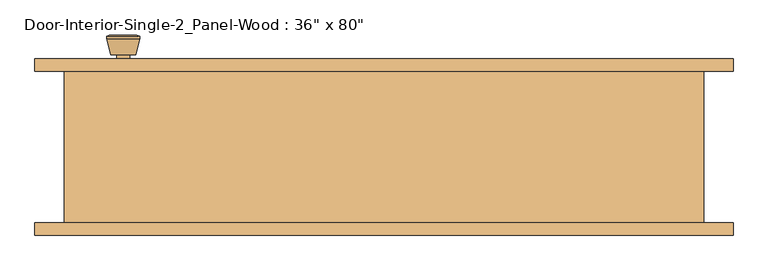
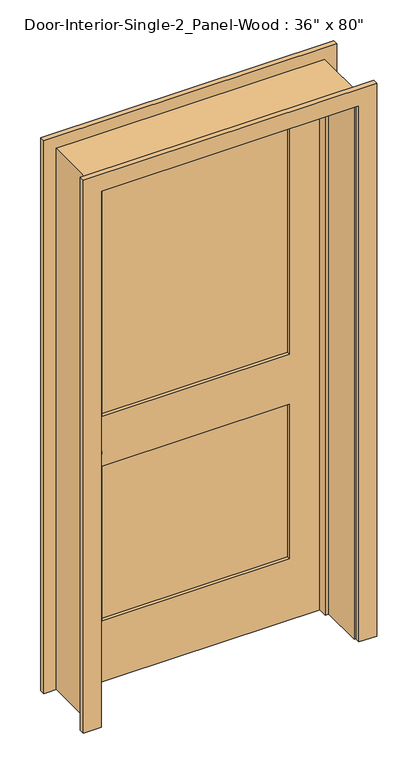
"""IFC4 building model written with IfcOpenShell, lengths in millimetres: door geometry."""

from ifc_helpers import new_model, si_unit, point, frame, frame_2d, origin, place, context, project, spatial, polyline, circle_curve, trimmed, segment, composite_curve, outline, extrude, faceted_brep, source, transform, mapped, element, save
from ifc_brep_helpers import plane_surface, cylinder_surface, revolved_surface, advanced_brep


def door_18b56f29(model_context):
    return source(origin(), model_context, "Body", "SolidModel", [
        advanced_brep(
        [(-393.7, 70.2, 914.4), (-383.7, 70.2, 914.4), (-403.7, 70.2, 914.4), (-373.2241324, 21.2, 914.4), (-393.7, 21.2, 914.4), (-414.1758676, 21.2, 914.4), (-368.7, 23.0278681, 914.4), (-418.7, 23.0278681, 914.4), (-368.7, 26.4915463, 914.4), (-418.7, 26.4915463, 914.4), (-375.063764, 51.2, 914.4), (-412.336236, 51.2, 914.4), (-383.7, 51.2, 914.4), (-403.7, 51.2, 914.4)],
        [
            (0, 1),
            (1, 2, circle_curve(frame((-393.7, 70.2, 914.4), z_axis=(0.0, 1.0, 0.0), x_axis=(-1.0, 0.0, 0.0)), 10.0)),
            (2, 0),
            (2, 1, circle_curve(frame((-393.7, 70.2, 914.4), z_axis=(0.0, 1.0, 0.0), x_axis=(-1.0, 0.0, 0.0)), 10.0)),
            (3, 4),
            (4, 5),
            (5, 3, circle_curve(frame((-393.7, 21.2, 914.4), z_axis=(0.0, -1.0, 0.0), x_axis=(-1.0, 0.0, 0.0)), 20.4758676)),
            (3, 5, circle_curve(frame((-393.7, 21.2, 914.4), z_axis=(0.0, -1.0, 0.0), x_axis=(-1.0, 0.0, 0.0)), 20.4758676)),
            (6, 3),
            (5, 7),
            (7, 6, circle_curve(frame((-393.7, 23.0278681, 914.4), z_axis=(0.0, -1.0, 0.0), x_axis=(-1.0, 0.0, 0.0)), 25.0)),
            (6, 7, circle_curve(frame((-393.7, 23.0278681, 914.4), z_axis=(0.0, -1.0, 0.0), x_axis=(-1.0, 0.0, 0.0)), 25.0)),
            (8, 6),
            (7, 9),
            (9, 8, circle_curve(frame((-393.7, 26.4915463, 914.4), z_axis=(0.0, -1.0, 0.0), x_axis=(-1.0, 0.0, 0.0)), 25.0)),
            (8, 9, circle_curve(frame((-393.7, 26.4915463, 914.4), z_axis=(0.0, -1.0, 0.0), x_axis=(-1.0, 0.0, 0.0)), 25.0)),
            (10, 8),
            (9, 11),
            (11, 10, circle_curve(frame((-393.7, 51.2, 914.4), z_axis=(0.0, -1.0, 0.0), x_axis=(-1.0, 0.0, 0.0)), 18.636236)),
            (10, 11, circle_curve(frame((-393.7, 51.2, 914.4), z_axis=(0.0, -1.0, 0.0), x_axis=(-1.0, 0.0, 0.0)), 18.636236)),
            (12, 10),
            (11, 13),
            (13, 12, circle_curve(frame((-393.7, 51.2, 914.4), z_axis=(0.0, -1.0, 0.0), x_axis=(-1.0, 0.0, 0.0)), 10.0)),
            (12, 13, circle_curve(frame((-393.7, 51.2, 914.4), z_axis=(0.0, -1.0, 0.0), x_axis=(-1.0, 0.0, 0.0)), 10.0)),
            (1, 12),
            (13, 2),
        ],
        [
            plane_surface(frame((-393.7, 70.2, 914.4), z_axis=(0.0, 1.0, 0.0), x_axis=(-1.0, 0.0, 0.0))),
            plane_surface(frame((-393.7, 21.2, 914.4), z_axis=(0.0, -1.0, 0.0), x_axis=(-1.0, 0.0, 0.0))),
            revolved_surface(polyline([(-414.1758676, 21.2, 914.4), (-418.7, 23.0278681, 914.4)]), (-393.7, 70.2, 914.4), (0.0, 1.0, 0.0)),
            cylinder_surface(frame((-393.7, 70.2, 914.4), z_axis=(0.0, 1.0, 0.0), x_axis=(-1.0, 0.0, 0.0)), 25.0),
            revolved_surface(polyline([(-418.7, 26.4915463, 914.4), (-412.336236, 51.2, 914.4)]), (-393.7, 70.2, 914.4), (0.0, 1.0, 0.0)),
            plane_surface(frame((-393.7, 51.2, 914.4), z_axis=(0.0, 1.0, 0.0), x_axis=(-1.0, 0.0, 0.0))),
            cylinder_surface(frame((-393.7, 70.2, 914.4), z_axis=(0.0, 1.0, 0.0), x_axis=(-1.0, 0.0, 0.0)), 10.0),
        ],
        [
            (0, [[1, 2, 3]]),
            (0, [[-3, 4, -1]]),
            (1, [[5, 6, 7]]),
            (1, [[-6, -5, 8]]),
            (2, [[9, -7, 10, 11]]),
            (2, [[-10, -8, -9, 12]]),
            (3, [[13, -11, 14, 15]]),
            (3, [[-14, -12, -13, 16]]),
            (4, [[17, -15, 18, 19]]),
            (4, [[-18, -16, -17, 20]]),
            (5, [[21, -19, 22, 23]]),
            (5, [[-22, -20, -21, 24]]),
            (6, [[25, -23, 26, -2]]),
            (6, [[-26, -24, -25, -4]]),
        ],
    ),
        extrude(outline(composite_curve([segment(trimmed(circle_curve(frame_2d((914.4, -393.7)), 30.0), [point((914.4, -423.7))], [point((914.4, -363.7))], False, "CARTESIAN"), True, "CONTINUOUS"), segment(trimmed(circle_curve(frame_2d((914.4, -393.7)), 30.0), [point((914.4, -363.7))], [point((914.4, -423.7))], False, "CARTESIAN"), True, "CONTINUOUS")], self_intersect=False)), frame((0.0, 70.2, 0.0), z_axis=(0.0, 1.0, 0.0), x_axis=(0.0, 0.0, 1.0)), (0.0, 0.0, 1.0), 6.0),
        advanced_brep(
        [(-393.7, 117.125, 914.4), (-403.7, 117.125, 914.4), (-383.7, 117.125, 914.4), (-373.2241324, 166.125, 914.4), (-414.1758676, 166.125, 914.4), (-393.7, 166.125, 914.4), (-368.7, 164.2971319, 914.4), (-418.7, 164.2971319, 914.4), (-368.7, 160.8334537, 914.4), (-418.7, 160.8334537, 914.4), (-375.063764, 136.125, 914.4), (-412.336236, 136.125, 914.4), (-383.7, 136.125, 914.4), (-403.7, 136.125, 914.4)],
        [
            (0, 1),
            (1, 2, circle_curve(frame((-393.7, 117.125, 914.4), z_axis=(0.0, -1.0, 0.0), x_axis=(-1.0, 0.0, 0.0)), 10.0)),
            (2, 0),
            (2, 1, circle_curve(frame((-393.7, 117.125, 914.4), z_axis=(0.0, -1.0, 0.0), x_axis=(-1.0, 0.0, 0.0)), 10.0)),
            (3, 4, circle_curve(frame((-393.7, 166.125, 914.4), z_axis=(0.0, 1.0, 0.0), x_axis=(-1.0, 0.0, 0.0)), 20.4758676)),
            (4, 5),
            (5, 3),
            (4, 3, circle_curve(frame((-393.7, 166.125, 914.4), z_axis=(0.0, 1.0, 0.0), x_axis=(-1.0, 0.0, 0.0)), 20.4758676)),
            (6, 7, circle_curve(frame((-393.7, 164.2971319, 914.4), z_axis=(0.0, 1.0, 0.0), x_axis=(-1.0, 0.0, 0.0)), 25.0)),
            (7, 4),
            (3, 6),
            (7, 6, circle_curve(frame((-393.7, 164.2971319, 914.4), z_axis=(0.0, 1.0, 0.0), x_axis=(-1.0, 0.0, 0.0)), 25.0)),
            (8, 9, circle_curve(frame((-393.7, 160.8334537, 914.4), z_axis=(0.0, 1.0, 0.0), x_axis=(-1.0, 0.0, 0.0)), 25.0)),
            (9, 7),
            (6, 8),
            (9, 8, circle_curve(frame((-393.7, 160.8334537, 914.4), z_axis=(0.0, 1.0, 0.0), x_axis=(-1.0, 0.0, 0.0)), 25.0)),
            (10, 11, circle_curve(frame((-393.7, 136.125, 914.4), z_axis=(0.0, 1.0, 0.0), x_axis=(-1.0, 0.0, 0.0)), 18.636236)),
            (11, 9),
            (8, 10),
            (11, 10, circle_curve(frame((-393.7, 136.125, 914.4), z_axis=(0.0, 1.0, 0.0), x_axis=(-1.0, 0.0, 0.0)), 18.636236)),
            (12, 13, circle_curve(frame((-393.7, 136.125, 914.4), z_axis=(0.0, 1.0, 0.0), x_axis=(-1.0, 0.0, 0.0)), 10.0)),
            (13, 11),
            (10, 12),
            (13, 12, circle_curve(frame((-393.7, 136.125, 914.4), z_axis=(0.0, 1.0, 0.0), x_axis=(-1.0, 0.0, 0.0)), 10.0)),
            (1, 13),
            (12, 2),
        ],
        [
            plane_surface(frame((-393.7, 117.125, 914.4), z_axis=(0.0, -1.0, 0.0), x_axis=(-1.0, 0.0, 0.0))),
            plane_surface(frame((-393.7, 166.125, 914.4), z_axis=(0.0, 1.0, 0.0), x_axis=(-1.0, 0.0, 0.0))),
            revolved_surface(polyline([(-414.1758676, 166.125, 914.4), (-418.7, 164.2971319, 914.4)]), (-393.7, 117.125, 914.4), (0.0, -1.0, 0.0)),
            cylinder_surface(frame((-393.7, 117.125, 914.4), z_axis=(0.0, -1.0, 0.0), x_axis=(-1.0, 0.0, 0.0)), 25.0),
            revolved_surface(polyline([(-418.7, 160.8334537, 914.4), (-412.336236, 136.125, 914.4)]), (-393.7, 117.125, 914.4), (0.0, -1.0, 0.0)),
            plane_surface(frame((-393.7, 136.125, 914.4), z_axis=(0.0, -1.0, 0.0), x_axis=(-1.0, 0.0, 0.0))),
            cylinder_surface(frame((-393.7, 117.125, 914.4), z_axis=(0.0, -1.0, 0.0), x_axis=(-1.0, 0.0, 0.0)), 10.0),
        ],
        [
            (0, [[1, 2, 3]]),
            (0, [[-3, 4, -1]]),
            (1, [[5, 6, 7]]),
            (1, [[8, -7, -6]]),
            (2, [[9, 10, -5, 11]]),
            (2, [[12, -11, -8, -10]]),
            (3, [[13, 14, -9, 15]]),
            (3, [[16, -15, -12, -14]]),
            (4, [[17, 18, -13, 19]]),
            (4, [[20, -19, -16, -18]]),
            (5, [[21, 22, -17, 23]]),
            (5, [[24, -23, -20, -22]]),
            (6, [[-2, 25, -21, 26]]),
            (6, [[-4, -26, -24, -25]]),
        ],
    ),
        extrude(outline(composite_curve([segment(trimmed(circle_curve(frame_2d((914.4, -393.7)), 30.0), [point((914.4, -423.7))], [point((914.4, -363.7))], False, "CARTESIAN"), True, "CONTINUOUS"), segment(trimmed(circle_curve(frame_2d((914.4, -393.7)), 30.0), [point((914.4, -363.7))], [point((914.4, -423.7))], False, "CARTESIAN"), True, "CONTINUOUS")], self_intersect=False)), frame((0.0, 111.125, 0.0), z_axis=(0.0, 1.0, 0.0), x_axis=(0.0, 0.0, 1.0)), (0.0, 0.0, 1.0), 6.0),
        faceted_brep([(482.6, 111.125, 0.0), (482.6, -117.475, 0.0), (457.2, -117.475, 0.0), (457.2, 41.275, 0.0), (444.5, 41.275, 0.0), (444.5, 76.2, 0.0), (457.2, 76.2, 0.0), (457.2, 111.125, 0.0), (482.6, 111.125, 2057.4), (482.6, -117.475, 2057.4), (-482.6, -117.475, 2057.4), (-482.6, -117.475, 0.0), (-457.2, -117.475, 0.0), (-457.2, -117.475, 2032.0), (457.2, -117.475, 2032.0), (457.2, 41.275, 2032.0), (-457.2, 41.275, 2032.0), (-457.2, 41.275, 0.0), (-444.5, 41.275, 0.0), (-444.5, 41.275, 2019.3), (444.5, 41.275, 2019.3), (444.5, 76.2, 2019.3), (-444.5, 76.2, 2019.3), (-444.5, 76.2, 0.0), (-457.2, 76.2, 0.0), (-457.2, 76.2, 2032.0), (457.2, 76.2, 2032.0), (457.2, 111.125, 2032.0), (-457.2, 111.125, 2032.0), (-457.2, 111.125, 0.0), (-482.6, 111.125, 0.0), (-482.6, 111.125, 2057.4)], [[[0, 1, 2, 3, 4, 5, 6, 7]], [[1, 0, 8, 9]], [[2, 1, 9, 10, 11, 12, 13, 14]], [[3, 2, 14, 15]], [[4, 3, 15, 16, 17, 18, 19, 20]], [[5, 4, 20, 21]], [[6, 5, 21, 22, 23, 24, 25, 26]], [[7, 6, 26, 27]], [[0, 7, 27, 28, 29, 30, 31, 8]], [[9, 8, 31, 10]], [[15, 14, 13, 16]], [[21, 20, 19, 22]], [[27, 26, 25, 28]], [[30, 29, 24, 23, 18, 17, 12, 11]], [[10, 31, 30, 11]], [[16, 13, 12, 17]], [[22, 19, 18, 23]], [[28, 25, 24, 29]]]),
        extrude(outline(polyline([(2032.0, -457.2), (0.0, -457.2), (0.0, 457.2), (2032.0, 457.2), (2032.0, -457.2)]), holes=[polyline([(1912.9375, -336.55), (1912.9375, 336.55), (1009.65, 336.55), (1009.65, -336.55), (1912.9375, -336.55)]), polyline([(819.15, -336.55), (819.15, 336.55), (231.775, 336.55), (231.775, -336.55), (819.15, -336.55)])]), frame((0.0, 76.2, 0.0), z_axis=(0.0, 1.0, 0.0), x_axis=(0.0, 0.0, 1.0)), (0.0, 0.0, 1.0), 34.925),
        extrude(outline(polyline([(336.55, 87.8416667), (-336.55, 87.8416667), (-336.55, 99.4833333), (336.55, 99.4833333), (336.55, 87.8416667)])), frame((0.0, 0.0, 1009.65), z_axis=(0.0, 0.0, 1.0), x_axis=(1.0, 0.0, 0.0)), (0.0, 0.0, 1.0), 903.2875),
        extrude(outline(polyline([(336.55, 87.8416667), (-336.55, 87.8416667), (-336.55, 99.4833333), (336.55, 99.4833333), (336.55, 87.8416667)])), frame((0.0, 0.0, 231.775), z_axis=(0.0, 0.0, 1.0), x_axis=(1.0, 0.0, 0.0)), (0.0, 0.0, 1.0), 587.375),
        extrude(outline(polyline([(0.0, 463.55), (0.0, 527.05), (2101.85, 527.05), (2101.85, -527.05), (0.0, -527.05), (0.0, -463.55), (2038.35, -463.55), (2038.35, 463.55), (0.0, 463.55)])), frame((0.0, 111.125, 0.0), z_axis=(0.0, 1.0, 0.0), x_axis=(0.0, 0.0, 1.0)), (0.0, 0.0, 1.0), 19.05),
        extrude(outline(polyline([(0.0, 463.55), (0.0, 527.05), (2101.85, 527.05), (2101.85, -527.05), (0.0, -527.05), (0.0, -463.55), (2038.35, -463.55), (2038.35, 463.55), (0.0, 463.55)])), frame((0.0, -136.525, 0.0), z_axis=(0.0, 1.0, 0.0), x_axis=(0.0, 0.0, 1.0)), (0.0, 0.0, 1.0), 19.05),
    ])


if __name__ == "__main__":
    model = new_model("IFC4")
    model_context = context("Model", 3, world=origin())
    ifc_project = project(units=[si_unit("LENGTHUNIT", "METRE", prefix="MILLI")], contexts=[model_context])
    site = spatial("IfcSite", under=ifc_project)
    building = spatial("IfcBuilding", under=site)
    placement = place(None, origin())
    door_shape = door_18b56f29(model_context)
    element("IfcDoor", 1, ObjectType="Door-Interior-Single-2_Panel-Wood : 36\" x 80\"", at=placement, inside=building, context=model_context, shape_type="MappedRepresentation", body=[
        mapped(door_shape, transform((0.0, 0.0, 0.0), x_axis=(1.0, 0.0, 0.0), y_axis=(0.0, 1.0, 0.0), z_axis=(0.0, 0.0, 1.0))),
    ])
    save(model, "model.ifc")

# Revit data of these elements
# Type "Door-Interior-Single-2_Panel-Wood : 36\" x 80\""
#   Type Mark = "8"
#   Assembly Code = "C1020300"
#   Analytic Construction = "Wooden"
#   Top Rail = 0' - 4 11/16"
#   Thickness = 0' - 1 3/8"
#   Thermal Resistance (R) = 2.5876 (h·ft²·°F)/BTU
#   Swing Angle [instance default] = 90.00°
#   Stiles = 0' - 4 3/4"
#   Rough Width = 3' - 2"
#   Rough Height = 6' - 9"
#   Lock Rail = 0' - 7 1/2"
#   Height = 6' - 8"
#   Width = 3' - 0"
#   Heat Transfer Coefficient (U) = 0.3865 BTU/(h·ft²·°F)
#   Bottom Rail = 0' - 9 1/8"
#   Trim Material = Cherry
#   Panel Material = Cherry
#   Frame Material = Cherry
#   Door Handle Material = Aluminum
#   Visual Light Transmittance = 0
#   Solar Heat Gain Coefficient = 0
#   Wall Closure = (empty or 0)
#   Function = (empty or 0)
# Element 1 (IfcDoor, "Door-Interior-Single-2_Panel-Wood : 36\" x 80\"")
#   Materials on its faces: "Cherry", "Aluminum"
# Materials
#   "Cherry": class "Wood", colour RGB 226 177 128, transparency 0, Description = "Prunus Serotina", Cost = 0
#   "Aluminum": class "Metal", colour RGB 247 247 247, transparency 0, Description = "Aluminum 6061", Cost = 0
